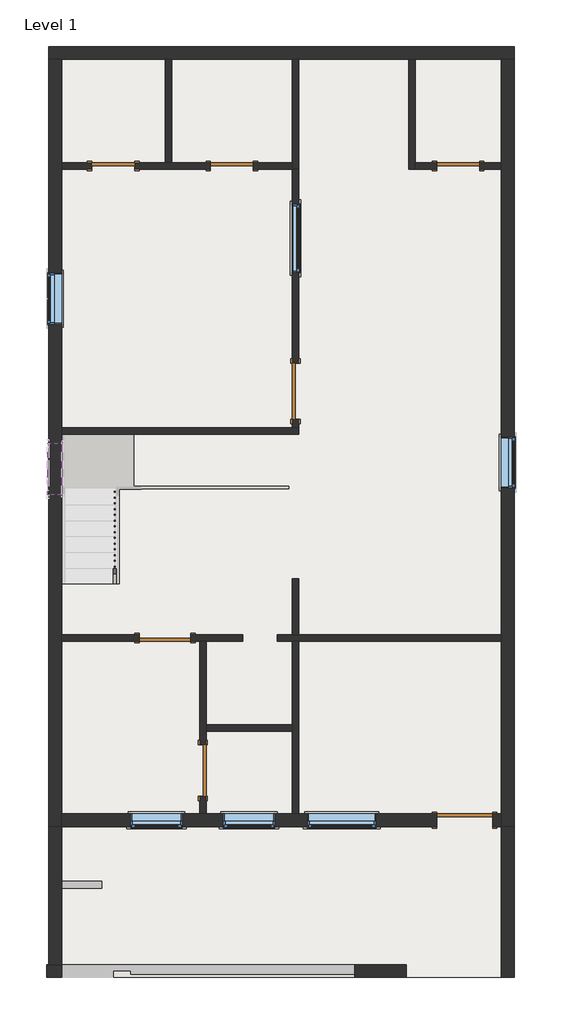
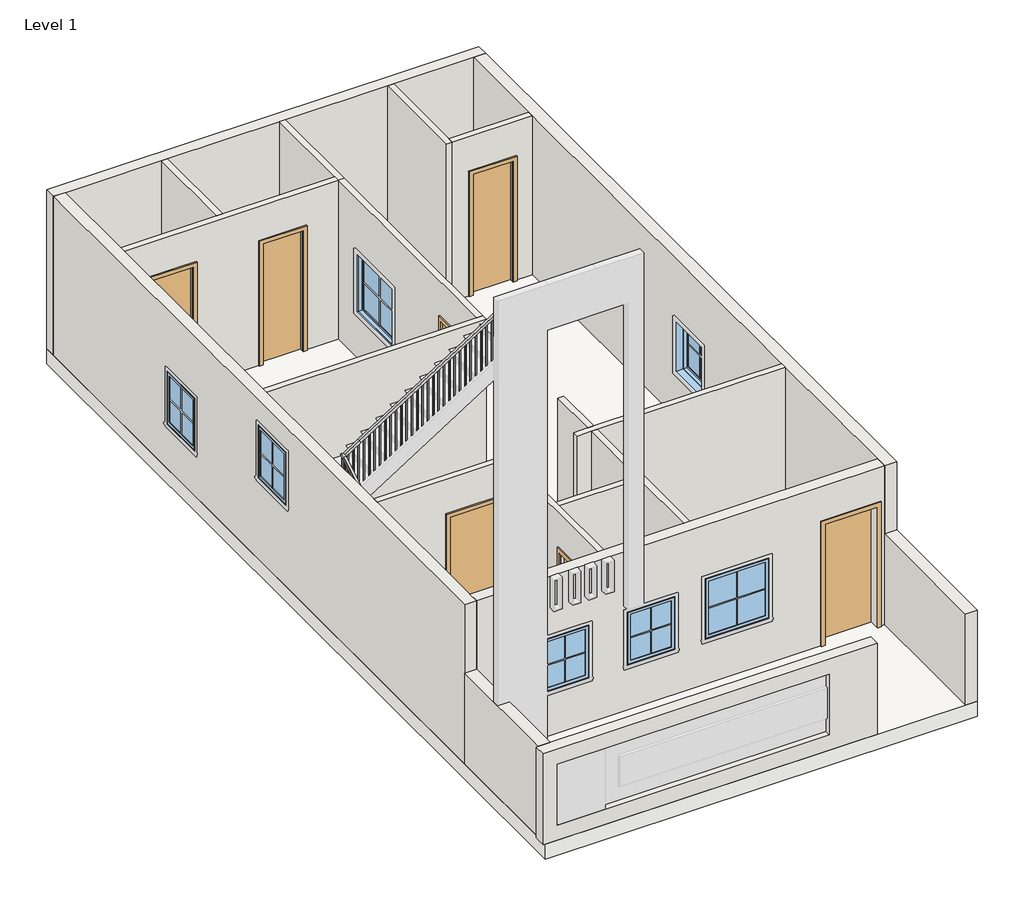
# One storey, part 1 of 2: 19 walls, 7 doors, 7 windows, 1 railing, 1 slab.
"""IFC4 building model written with IfcOpenShell, lengths in millimetres."""

from ifc_helpers import new_model, si_unit, frame, origin, origin_with_axes, place, context, project, spatial, polyline, outline, extrude, faceted_brep, transform, mapped, element, save
from components import door_02e7543a, door_3ddad2be, single_flush_d2_3_x_7_58d0fc15, door_c9b15bbd, door_019bc352, window_casement_single_left_w_4_x_4_e869003f, window_casement_single_left_w_4_x_4_9640c864, window_cb922c77, window_a1546d9a

model = new_model("IFC4")

# Units and contexts
model_context = context("Model", 3, world=origin())
ifc_project = project(units=[si_unit("LENGTHUNIT", "METRE", prefix="MILLI")], contexts=[model_context])

# Site, building, storey
site = spatial("IfcSite", under=ifc_project)
building = spatial("IfcBuilding", under=site)
storey = spatial("IfcBuildingStorey", under=building, Name="Level 1", Elevation=0.0)

# Doors
placement = place(None, origin())
door_shape = door_02e7543a(model_context)
element("IfcDoor", 1, ObjectType="Single-Flush : D1 3'3\" X 7'", at=placement, inside=storey, context=model_context, shape_type="MappedRepresentation", body=[
    mapped(door_shape, transform((-6568.6167709, -3138.8637867, 0.0), x_axis=(1.0, 0.0, 0.0), y_axis=(0.0, 1.0, 0.0), z_axis=(0.0, 0.0, 1.0))),
])
door_2_shape = door_3ddad2be(model_context)
element("IfcDoor", 2, ObjectType="Single-Flush : D1 3'3\" X 7'", at=placement, inside=storey, context=model_context, shape_type="MappedRepresentation", body=[
    mapped(door_2_shape, transform((-9559.4667709, 4443.0362133, 0.0), x_axis=(0.0, -1.0, 0.0), y_axis=(1.0, 0.0, 0.0), z_axis=(0.0, 0.0, 1.0))),
])
single_flush_d2_3_x_7_shape = single_flush_d2_3_x_7_58d0fc15(model_context)
element("IfcDoor", 3, ObjectType="Single-Flush : D2 3' X 7'", at=placement, inside=storey, context=model_context, shape_type="MappedRepresentation", body=[
    mapped(single_flush_d2_3_x_7_shape, transform((-11864.5167709, 80.5862133, 0.0), x_axis=(1.0, 0.0, 0.0), y_axis=(0.0, 1.0, 0.0), z_axis=(0.0, 0.0, 1.0))),
])
element("IfcDoor", 4, ObjectType="Single-Flush : D2 3' X 7'", at=placement, inside=storey, context=model_context, shape_type="MappedRepresentation", body=[
    mapped(single_flush_d2_3_x_7_shape, transform((-11197.7667709, -2262.5637867, 0.0), x_axis=(0.0, 1.0, 0.0), y_axis=(-1.0, 0.0, 0.0), z_axis=(0.0, 0.0, 1.0))),
])
door_3_shape = door_c9b15bbd(model_context)
element("IfcDoor", 5, ObjectType="Single-Flush : D3 2'6\" X 7'", at=placement, inside=storey, context=model_context, shape_type="MappedRepresentation", body=[
    mapped(door_3_shape, transform((-12778.9167709, 8424.4862133, 0.0), x_axis=(1.0, 0.0, 0.0), y_axis=(0.0, 1.0, 0.0), z_axis=(0.0, 0.0, 1.0))),
])
door_4_shape = door_019bc352(model_context)
element("IfcDoor", 6, ObjectType="Single-Flush : D3 2'6\" X 7'", at=placement, inside=storey, context=model_context, shape_type="MappedRepresentation", body=[
    mapped(door_4_shape, transform((-10683.4167709, 8424.4862133, 0.0), x_axis=(-1.0, 0.0, 0.0), y_axis=(0.0, -1.0, 0.0), z_axis=(0.0, 0.0, 1.0))),
])
element("IfcDoor", 7, ObjectType="Single-Flush : D3 2'6\" X 7'", at=placement, inside=storey, context=model_context, shape_type="MappedRepresentation", body=[
    mapped(door_4_shape, transform((-6682.9167709, 8424.4862133, 0.0), x_axis=(-1.0, 0.0, 0.0), y_axis=(0.0, -1.0, 0.0), z_axis=(0.0, 0.0, 1.0))),
])

# Railing
element("IfcRailing", 8, ObjectType="Handrail - Rectangular", at=placement, inside=storey, context=model_context, shape_type="SolidModel", body=[
    faceted_brep([(-12778.9167709, 1039.4362133, 1092.2), (-12778.9167709, 1039.4362133, 1031.986276), (-12728.1167709, 1039.4362133, 1031.986276), (-12728.1167709, 1039.4362133, 1092.2), (-12778.9167709, 2715.8362133, 2159.0), (-12778.9167709, 2730.6292082, 2108.2), (-12728.1167709, 2730.6292082, 2108.2), (-12728.1167709, 2715.8362133, 2159.0), (-12778.9167709, 2817.4362133, 2159.0), (-12728.1167709, 2817.4362133, 2159.0), (-12728.1167709, 2817.4362133, 2108.2), (-12778.9167709, 2817.4362133, 2108.2)], [[[0, 1, 2, 3]], [[1, 0, 4, 5]], [[2, 1, 5, 6]], [[3, 2, 6, 7]], [[0, 3, 7, 4]], [[8, 9, 10, 11]], [[5, 4, 8, 11]], [[6, 5, 11, 10]], [[7, 6, 10, 9]], [[4, 7, 9, 8]]]),
    faceted_brep([(-12728.1167709, 2817.4362133, 2159.0), (-12728.1167709, 2817.4362133, 2098.786276), (-12728.1167709, 2766.6362133, 2098.786276), (-12728.1167709, 2766.6362133, 2159.0), (-12448.7167709, 2817.4362133, 2336.8), (-12421.4434959, 2817.4362133, 2293.9419964), (-12421.4434959, 2766.6362133, 2293.9419964), (-12448.7167709, 2766.6362133, 2336.8), (-9654.7167709, 2817.4362133, 4114.8), (-9654.7167709, 2766.6362133, 4114.8), (-9654.7167709, 2766.6362133, 4054.586276), (-9654.7167709, 2817.4362133, 4054.586276)], [[[0, 1, 2, 3]], [[1, 0, 4, 5]], [[2, 1, 5, 6]], [[3, 2, 6, 7]], [[0, 3, 7, 4]], [[8, 9, 10, 11]], [[5, 4, 8, 11]], [[6, 5, 11, 10]], [[7, 6, 10, 9]], [[4, 7, 9, 8]]]),
    extrude(outline(polyline([(4028.3203669, -9695.9917709), (4016.1976396, -9715.0417709), (3022.6, -9715.0417709), (3022.6, -9695.9917709), (4028.3203669, -9695.9917709)])), frame((0.0, 2782.5112133, 0.0), z_axis=(0.0, 1.0, 0.0), x_axis=(0.0, 0.0, 1.0)), (0.0, 0.0, 1.0), 19.05),
    extrude(outline(polyline([(3963.6658214, -9797.5917709), (3951.5430941, -9816.6417709), (3022.6, -9816.6417709), (3022.6, -9797.5917709), (3963.6658214, -9797.5917709)])), frame((0.0, 2782.5112133, 0.0), z_axis=(0.0, 1.0, 0.0), x_axis=(0.0, 0.0, 1.0)), (0.0, 0.0, 1.0), 19.05),
    extrude(outline(polyline([(3899.011276, -9899.1917709), (3886.8885487, -9918.2417709), (3022.6, -9918.2417709), (3022.6, -9899.1917709), (3899.011276, -9899.1917709)])), frame((0.0, 2782.5112133, 0.0), z_axis=(0.0, 1.0, 0.0), x_axis=(0.0, 0.0, 1.0)), (0.0, 0.0, 1.0), 19.05),
    extrude(outline(polyline([(3834.3567305, -10000.7917709), (3822.2340032, -10019.8417709), (2844.8, -10019.8417709), (2844.8, -10000.7917709), (3834.3567305, -10000.7917709)])), frame((0.0, 2782.5112133, 0.0), z_axis=(0.0, 1.0, 0.0), x_axis=(0.0, 0.0, 1.0)), (0.0, 0.0, 1.0), 19.05),
    extrude(outline(polyline([(3769.7021851, -10102.3917709), (3757.5794578, -10121.4417709), (2844.8, -10121.4417709), (2844.8, -10102.3917709), (3769.7021851, -10102.3917709)])), frame((0.0, 2782.5112133, 0.0), z_axis=(0.0, 1.0, 0.0), x_axis=(0.0, 0.0, 1.0)), (0.0, 0.0, 1.0), 19.05),
    extrude(outline(polyline([(3705.0476396, -10203.9917709), (3692.9249123, -10223.0417709), (2844.8, -10223.0417709), (2844.8, -10203.9917709), (3705.0476396, -10203.9917709)])), frame((0.0, 2782.5112133, 0.0), z_axis=(0.0, 1.0, 0.0), x_axis=(0.0, 0.0, 1.0)), (0.0, 0.0, 1.0), 19.05),
    extrude(outline(polyline([(3640.3930941, -10305.5917709), (3628.2703669, -10324.6417709), (2667.0, -10324.6417709), (2667.0, -10305.5917709), (3640.3930941, -10305.5917709)])), frame((0.0, 2782.5112133, 0.0), z_axis=(0.0, 1.0, 0.0), x_axis=(0.0, 0.0, 1.0)), (0.0, 0.0, 1.0), 19.05),
    extrude(outline(polyline([(3575.7385487, -10407.1917709), (3563.6158214, -10426.2417709), (2667.0, -10426.2417709), (2667.0, -10407.1917709), (3575.7385487, -10407.1917709)])), frame((0.0, 2782.5112133, 0.0), z_axis=(0.0, 1.0, 0.0), x_axis=(0.0, 0.0, 1.0)), (0.0, 0.0, 1.0), 19.05),
    extrude(outline(polyline([(3511.0840032, -10508.7917709), (3498.961276, -10527.8417709), (2489.2, -10527.8417709), (2489.2, -10508.7917709), (3511.0840032, -10508.7917709)])), frame((0.0, 2782.5112133, 0.0), z_axis=(0.0, 1.0, 0.0), x_axis=(0.0, 0.0, 1.0)), (0.0, 0.0, 1.0), 19.05),
    extrude(outline(polyline([(3446.4294578, -10610.3917709), (3434.3067305, -10629.4417709), (2489.2, -10629.4417709), (2489.2, -10610.3917709), (3446.4294578, -10610.3917709)])), frame((0.0, 2782.5112133, 0.0), z_axis=(0.0, 1.0, 0.0), x_axis=(0.0, 0.0, 1.0)), (0.0, 0.0, 1.0), 19.05),
    extrude(outline(polyline([(3381.7749123, -10711.9917709), (3369.6521851, -10731.0417709), (2489.2, -10731.0417709), (2489.2, -10711.9917709), (3381.7749123, -10711.9917709)])), frame((0.0, 2782.5112133, 0.0), z_axis=(0.0, 1.0, 0.0), x_axis=(0.0, 0.0, 1.0)), (0.0, 0.0, 1.0), 19.05),
    extrude(outline(polyline([(3317.1203669, -10813.5917709), (3304.9976396, -10832.6417709), (2311.4, -10832.6417709), (2311.4, -10813.5917709), (3317.1203669, -10813.5917709)])), frame((0.0, 2782.5112133, 0.0), z_axis=(0.0, 1.0, 0.0), x_axis=(0.0, 0.0, 1.0)), (0.0, 0.0, 1.0), 19.05),
    extrude(outline(polyline([(3252.4658214, -10915.1917709), (3240.3430941, -10934.2417709), (2311.4, -10934.2417709), (2311.4, -10915.1917709), (3252.4658214, -10915.1917709)])), frame((0.0, 2782.5112133, 0.0), z_axis=(0.0, 1.0, 0.0), x_axis=(0.0, 0.0, 1.0)), (0.0, 0.0, 1.0), 19.05),
    extrude(outline(polyline([(3187.811276, -11016.7917709), (3175.6885487, -11035.8417709), (2311.4, -11035.8417709), (2311.4, -11016.7917709), (3187.811276, -11016.7917709)])), frame((0.0, 2782.5112133, 0.0), z_axis=(0.0, 1.0, 0.0), x_axis=(0.0, 0.0, 1.0)), (0.0, 0.0, 1.0), 19.05),
    extrude(outline(polyline([(3123.1567305, -11118.3917709), (3111.0340032, -11137.4417709), (2133.6, -11137.4417709), (2133.6, -11118.3917709), (3123.1567305, -11118.3917709)])), frame((0.0, 2782.5112133, 0.0), z_axis=(0.0, 1.0, 0.0), x_axis=(0.0, 0.0, 1.0)), (0.0, 0.0, 1.0), 19.05),
    extrude(outline(polyline([(3058.5021851, -11219.9917709), (3046.3794578, -11239.0417709), (2133.6, -11239.0417709), (2133.6, -11219.9917709), (3058.5021851, -11219.9917709)])), frame((0.0, 2782.5112133, 0.0), z_axis=(0.0, 1.0, 0.0), x_axis=(0.0, 0.0, 1.0)), (0.0, 0.0, 1.0), 19.05),
    extrude(outline(polyline([(2993.8476396, -11321.5917709), (2981.7249123, -11340.6417709), (2133.6, -11340.6417709), (2133.6, -11321.5917709), (2993.8476396, -11321.5917709)])), frame((0.0, 2782.5112133, 0.0), z_axis=(0.0, 1.0, 0.0), x_axis=(0.0, 0.0, 1.0)), (0.0, 0.0, 1.0), 19.05),
    extrude(outline(polyline([(2929.1930941, -11423.1917709), (2917.0703669, -11442.2417709), (1955.8, -11442.2417709), (1955.8, -11423.1917709), (2929.1930941, -11423.1917709)])), frame((0.0, 2782.5112133, 0.0), z_axis=(0.0, 1.0, 0.0), x_axis=(0.0, 0.0, 1.0)), (0.0, 0.0, 1.0), 19.05),
    extrude(outline(polyline([(2864.5385487, -11524.7917709), (2852.4158214, -11543.8417709), (1955.8, -11543.8417709), (1955.8, -11524.7917709), (2864.5385487, -11524.7917709)])), frame((0.0, 2782.5112133, 0.0), z_axis=(0.0, 1.0, 0.0), x_axis=(0.0, 0.0, 1.0)), (0.0, 0.0, 1.0), 19.05),
    extrude(outline(polyline([(2799.8840032, -11626.3917709), (2787.761276, -11645.4417709), (1778.0, -11645.4417709), (1778.0, -11626.3917709), (2799.8840032, -11626.3917709)])), frame((0.0, 2782.5112133, 0.0), z_axis=(0.0, 1.0, 0.0), x_axis=(0.0, 0.0, 1.0)), (0.0, 0.0, 1.0), 19.05),
    extrude(outline(polyline([(2735.2294578, -11727.9917709), (2723.1067305, -11747.0417709), (1778.0, -11747.0417709), (1778.0, -11727.9917709), (2735.2294578, -11727.9917709)])), frame((0.0, 2782.5112133, 0.0), z_axis=(0.0, 1.0, 0.0), x_axis=(0.0, 0.0, 1.0)), (0.0, 0.0, 1.0), 19.05),
    extrude(outline(polyline([(2670.5749123, -11829.5917709), (2658.4521851, -11848.6417709), (1778.0, -11848.6417709), (1778.0, -11829.5917709), (2670.5749123, -11829.5917709)])), frame((0.0, 2782.5112133, 0.0), z_axis=(0.0, 1.0, 0.0), x_axis=(0.0, 0.0, 1.0)), (0.0, 0.0, 1.0), 19.05),
    extrude(outline(polyline([(2605.9203669, -11931.1917709), (2593.7976396, -11950.2417709), (1600.2, -11950.2417709), (1600.2, -11931.1917709), (2605.9203669, -11931.1917709)])), frame((0.0, 2782.5112133, 0.0), z_axis=(0.0, 1.0, 0.0), x_axis=(0.0, 0.0, 1.0)), (0.0, 0.0, 1.0), 19.05),
    extrude(outline(polyline([(2541.2658214, -12032.7917709), (2529.1430941, -12051.8417709), (1600.2, -12051.8417709), (1600.2, -12032.7917709), (2541.2658214, -12032.7917709)])), frame((0.0, 2782.5112133, 0.0), z_axis=(0.0, 1.0, 0.0), x_axis=(0.0, 0.0, 1.0)), (0.0, 0.0, 1.0), 19.05),
    extrude(outline(polyline([(2476.611276, -12134.3917709), (2464.4885487, -12153.4417709), (1600.2, -12153.4417709), (1600.2, -12134.3917709), (2476.611276, -12134.3917709)])), frame((0.0, 2782.5112133, 0.0), z_axis=(0.0, 1.0, 0.0), x_axis=(0.0, 0.0, 1.0)), (0.0, 0.0, 1.0), 19.05),
    extrude(outline(polyline([(2411.9567305, -12235.9917709), (2399.8340032, -12255.0417709), (1422.4, -12255.0417709), (1422.4, -12235.9917709), (2411.9567305, -12235.9917709)])), frame((0.0, 2782.5112133, 0.0), z_axis=(0.0, 1.0, 0.0), x_axis=(0.0, 0.0, 1.0)), (0.0, 0.0, 1.0), 19.05),
    extrude(outline(polyline([(2347.3021851, -12337.5917709), (2335.1794578, -12356.6417709), (1422.4, -12356.6417709), (1422.4, -12337.5917709), (2347.3021851, -12337.5917709)])), frame((0.0, 2782.5112133, 0.0), z_axis=(0.0, 1.0, 0.0), x_axis=(0.0, 0.0, 1.0)), (0.0, 0.0, 1.0), 19.05),
    extrude(outline(polyline([(2217.9930941, -12540.7917709), (2205.8703669, -12559.8417709), (1244.6, -12559.8417709), (1244.6, -12540.7917709), (2217.9930941, -12540.7917709)])), frame((0.0, 2782.5112133, 0.0), z_axis=(0.0, 1.0, 0.0), x_axis=(0.0, 0.0, 1.0)), (0.0, 0.0, 1.0), 19.05),
    extrude(outline(polyline([(2153.3385487, -12642.3917709), (2141.2158214, -12661.4417709), (1244.6, -12661.4417709), (1244.6, -12642.3917709), (2153.3385487, -12642.3917709)])), frame((0.0, 2782.5112133, 0.0), z_axis=(0.0, 1.0, 0.0), x_axis=(0.0, 0.0, 1.0)), (0.0, 0.0, 1.0), 19.05),
    extrude(outline(polyline([(2655.5112133, 2060.3976396), (2674.5612133, 2072.5203669), (2674.5612133, 1066.8), (2655.5112133, 1066.8), (2655.5112133, 2060.3976396)])), frame((-12763.0417709, 0.0, 0.0), z_axis=(1.0, 0.0, 0.0), x_axis=(0.0, 1.0, 0.0)), (0.0, 0.0, 1.0), 19.05),
    extrude(outline(polyline([(2553.9112133, 1995.7430941), (2572.9612133, 2007.8658214), (2572.9612133, 1066.8), (2553.9112133, 1066.8), (2553.9112133, 1995.7430941)])), frame((-12763.0417709, 0.0, 0.0), z_axis=(1.0, 0.0, 0.0), x_axis=(0.0, 1.0, 0.0)), (0.0, 0.0, 1.0), 19.05),
    extrude(outline(polyline([(2452.3112133, 1931.0885487), (2471.3612133, 1943.211276), (2471.3612133, 1066.8), (2452.3112133, 1066.8), (2452.3112133, 1931.0885487)])), frame((-12763.0417709, 0.0, 0.0), z_axis=(1.0, 0.0, 0.0), x_axis=(0.0, 1.0, 0.0)), (0.0, 0.0, 1.0), 19.05),
    extrude(outline(polyline([(2350.7112133, 1866.4340032), (2369.7612133, 1878.5567305), (2369.7612133, 889.0), (2350.7112133, 889.0), (2350.7112133, 1866.4340032)])), frame((-12763.0417709, 0.0, 0.0), z_axis=(1.0, 0.0, 0.0), x_axis=(0.0, 1.0, 0.0)), (0.0, 0.0, 1.0), 19.05),
    extrude(outline(polyline([(2249.1112133, 1801.7794578), (2268.1612133, 1813.9021851), (2268.1612133, 889.0), (2249.1112133, 889.0), (2249.1112133, 1801.7794578)])), frame((-12763.0417709, 0.0, 0.0), z_axis=(1.0, 0.0, 0.0), x_axis=(0.0, 1.0, 0.0)), (0.0, 0.0, 1.0), 19.05),
    extrude(outline(polyline([(2147.5112133, 1737.1249123), (2166.5612133, 1749.2476396), (2166.5612133, 889.0), (2147.5112133, 889.0), (2147.5112133, 1737.1249123)])), frame((-12763.0417709, 0.0, 0.0), z_axis=(1.0, 0.0, 0.0), x_axis=(0.0, 1.0, 0.0)), (0.0, 0.0, 1.0), 19.05),
    extrude(outline(polyline([(2045.9112133, 1672.4703669), (2064.9612133, 1684.5930941), (2064.9612133, 711.2), (2045.9112133, 711.2), (2045.9112133, 1672.4703669)])), frame((-12763.0417709, 0.0, 0.0), z_axis=(1.0, 0.0, 0.0), x_axis=(0.0, 1.0, 0.0)), (0.0, 0.0, 1.0), 19.05),
    extrude(outline(polyline([(1944.3112133, 1607.8158214), (1963.3612133, 1619.9385487), (1963.3612133, 711.2), (1944.3112133, 711.2), (1944.3112133, 1607.8158214)])), frame((-12763.0417709, 0.0, 0.0), z_axis=(1.0, 0.0, 0.0), x_axis=(0.0, 1.0, 0.0)), (0.0, 0.0, 1.0), 19.05),
    extrude(outline(polyline([(1842.7112133, 1543.161276), (1861.7612133, 1555.2840032), (1861.7612133, 533.4), (1842.7112133, 533.4), (1842.7112133, 1543.161276)])), frame((-12763.0417709, 0.0, 0.0), z_axis=(1.0, 0.0, 0.0), x_axis=(0.0, 1.0, 0.0)), (0.0, 0.0, 1.0), 19.05),
    extrude(outline(polyline([(1741.1112133, 1478.5067305), (1760.1612133, 1490.6294578), (1760.1612133, 533.4), (1741.1112133, 533.4), (1741.1112133, 1478.5067305)])), frame((-12763.0417709, 0.0, 0.0), z_axis=(1.0, 0.0, 0.0), x_axis=(0.0, 1.0, 0.0)), (0.0, 0.0, 1.0), 19.05),
    extrude(outline(polyline([(1639.5112133, 1413.8521851), (1658.5612133, 1425.9749123), (1658.5612133, 533.4), (1639.5112133, 533.4), (1639.5112133, 1413.8521851)])), frame((-12763.0417709, 0.0, 0.0), z_axis=(1.0, 0.0, 0.0), x_axis=(0.0, 1.0, 0.0)), (0.0, 0.0, 1.0), 19.05),
    extrude(outline(polyline([(1537.9112133, 1349.1976396), (1556.9612133, 1361.3203669), (1556.9612133, 355.6), (1537.9112133, 355.6), (1537.9112133, 1349.1976396)])), frame((-12763.0417709, 0.0, 0.0), z_axis=(1.0, 0.0, 0.0), x_axis=(0.0, 1.0, 0.0)), (0.0, 0.0, 1.0), 19.05),
    extrude(outline(polyline([(1436.3112133, 1284.5430941), (1455.3612133, 1296.6658214), (1455.3612133, 355.6), (1436.3112133, 355.6), (1436.3112133, 1284.5430941)])), frame((-12763.0417709, 0.0, 0.0), z_axis=(1.0, 0.0, 0.0), x_axis=(0.0, 1.0, 0.0)), (0.0, 0.0, 1.0), 19.05),
    extrude(outline(polyline([(1334.7112133, 1219.8885487), (1353.7612133, 1232.011276), (1353.7612133, 355.6), (1334.7112133, 355.6), (1334.7112133, 1219.8885487)])), frame((-12763.0417709, 0.0, 0.0), z_axis=(1.0, 0.0, 0.0), x_axis=(0.0, 1.0, 0.0)), (0.0, 0.0, 1.0), 19.05),
    extrude(outline(polyline([(1233.1112133, 1155.2340032), (1252.1612133, 1167.3567305), (1252.1612133, 177.8), (1233.1112133, 177.8), (1233.1112133, 1155.2340032)])), frame((-12763.0417709, 0.0, 0.0), z_axis=(1.0, 0.0, 0.0), x_axis=(0.0, 1.0, 0.0)), (0.0, 0.0, 1.0), 19.05),
    extrude(outline(polyline([(1131.5112133, 1090.5794578), (1150.5612133, 1102.7021851), (1150.5612133, 177.8), (1131.5112133, 177.8), (1131.5112133, 1090.5794578)])), frame((-12763.0417709, 0.0, 0.0), z_axis=(1.0, 0.0, 0.0), x_axis=(0.0, 1.0, 0.0)), (0.0, 0.0, 1.0), 19.05),
    extrude(outline(polyline([(2282.6476396, -12439.1917709), (2270.5249123, -12458.2417709), (1244.6, -12458.2417709), (1244.6, -12439.1917709), (2282.6476396, -12439.1917709)])), frame((0.0, 2782.5112133, 0.0), z_axis=(0.0, 1.0, 0.0), x_axis=(0.0, 0.0, 1.0)), (0.0, 0.0, 1.0), 19.05),
    extrude(outline(polyline([(-12743.9917709, 2782.5112133), (-12763.0417709, 2782.5112133), (-12763.0417709, 2801.5612133), (-12743.9917709, 2801.5612133), (-12743.9917709, 2782.5112133)])), frame((0.0, 0.0, 1244.6), z_axis=(0.0, 0.0, 1.0), x_axis=(1.0, 0.0, 0.0)), (0.0, 0.0, 1.0), 863.6),
    extrude(outline(polyline([(2706.3112133, 2092.7249123), (2725.3612133, 2104.8476396), (2725.3612133, 1244.6), (2706.3112133, 1244.6), (2706.3112133, 2092.7249123)])), frame((-12763.0417709, 0.0, 0.0), z_axis=(1.0, 0.0, 0.0), x_axis=(0.0, 1.0, 0.0)), (0.0, 0.0, 1.0), 19.05),
    extrude(outline(polyline([(4054.586276, -9654.7167709), (4042.4635487, -9673.7667709), (3022.6, -9673.7667709), (3022.6, -9654.7167709), (4054.586276, -9654.7167709)])), frame((0.0, 2782.5112133, 0.0), z_axis=(0.0, 1.0, 0.0), x_axis=(0.0, 0.0, 1.0)), (0.0, 0.0, 1.0), 19.05),
    extrude(outline(polyline([(1039.4362133, 1031.986276), (1058.4862133, 1044.1090032), (1058.4862133, 177.8), (1039.4362133, 177.8), (1039.4362133, 1031.986276)])), frame((-12763.0417709, 0.0, 0.0), z_axis=(1.0, 0.0, 0.0), x_axis=(0.0, 1.0, 0.0)), (0.0, 0.0, 1.0), 19.05),
])

# Slab
element("IfcSlab", 9, ObjectType="Generic - 12\"", at=placement, inside=storey, context=model_context, shape_type="SweptSolid", body=[
    extrude(outline(polyline([(-5692.3167709, 10539.0362133), (-5692.3167709, -5920.1637867), (-13921.9167709, -5920.1637867), (-13921.9167709, 10539.0362133), (-5692.3167709, 10539.0362133)])), frame((0.0, 0.0, -304.8), z_axis=(0.0, 0.0, 1.0), x_axis=(1.0, 0.0, 0.0)), (0.0, 0.0, 1.0), 304.8),
])

# Walls
element("IfcWall", 10, ObjectType="4.5\" inner wall", at=placement, inside=storey, context=model_context, shape_type="SweptSolid", body=[
    extrude(outline(polyline([(-11864.5167709, 8481.6362133), (-11864.5167709, 10310.4362133), (-11750.2167709, 10310.4362133), (-11750.2167709, 8481.6362133), (-11864.5167709, 8481.6362133)])), origin_with_axes(), (0.0, 0.0, 1.0), 3200.4),
])
element("IfcWall", 11, ObjectType="4.5\" inner wall", at=placement, inside=storey, context=model_context, shape_type="Brep", body=[
    faceted_brep([(-11064.4167709, 8481.6362133, 2438.4), (-11064.4167709, 8481.6362133, 0.0), (-11750.2167709, 8481.6362133, 0.0), (-11864.5167709, 8481.6362133, 0.0), (-12397.9167709, 8481.6362133, 0.0), (-12397.9167709, 8481.6362133, 2438.4), (-13159.9167709, 8481.6362133, 2438.4), (-13159.9167709, 8481.6362133, 0.0), (-13693.3167709, 8481.6362133, 0.0), (-13693.3167709, 8481.6362133, 3200.4), (-11864.5167709, 8481.6362133, 3200.4), (-11750.2167709, 8481.6362133, 3200.4), (-9616.6167709, 8481.6362133, 3200.4), (-9616.6167709, 8481.6362133, 0.0), (-10302.4167709, 8481.6362133, 0.0), (-10302.4167709, 8481.6362133, 2438.4), (-12397.9167709, 8367.3362133, 0.0), (-11064.4167709, 8367.3362133, 0.0), (-11064.4167709, 8367.3362133, 2438.4), (-10302.4167709, 8367.3362133, 2438.4), (-10302.4167709, 8367.3362133, 0.0), (-9616.6167709, 8367.3362133, 0.0), (-9616.6167709, 8367.3362133, 3200.4), (-13693.3167709, 8367.3362133, 3200.4), (-13693.3167709, 8367.3362133, 0.0), (-13159.9167709, 8367.3362133, 0.0), (-13159.9167709, 8367.3362133, 2438.4), (-12397.9167709, 8367.3362133, 2438.4)], [[[0, 1, 2, 3, 4, 5, 6, 7, 8, 9, 10, 11, 12, 13, 14, 15]], [[16, 17, 18, 19, 20, 21, 22, 23, 24, 25, 26, 27]], [[25, 24, 8, 7]], [[14, 13, 21, 20]], [[4, 3, 2, 1, 17, 16]], [[12, 11, 10, 9, 23, 22]], [[9, 8, 24, 23]], [[13, 12, 22, 21]], [[5, 4, 16, 27]], [[6, 5, 27, 26]], [[7, 6, 26, 25]], [[18, 17, 1, 0]], [[19, 18, 0, 15]], [[20, 19, 15, 14]]]),
])
element("IfcWall", 12, ObjectType="4.5\" inner wall", at=placement, inside=storey, context=model_context, shape_type="Brep", body=[
    faceted_brep([(-9616.6167709, 10310.4362133, 0.0), (-9616.6167709, 8481.6362133, 0.0), (-9616.6167709, 8367.3362133, 0.0), (-9616.6167709, 8367.3362133, 3200.4), (-9616.6167709, 8481.6362133, 3200.4), (-9616.6167709, 10310.4362133, 3200.4), (-9502.3167709, 10310.4362133, 0.0), (-9502.3167709, 10310.4362133, 3200.4), (-9502.3167709, 8367.3362133, 3200.4), (-9502.3167709, 8367.3362133, 0.0)], [[[0, 1, 2, 3, 4, 5]], [[6, 7, 8, 9]], [[2, 1, 0, 6, 9]], [[5, 4, 3, 8, 7]], [[0, 5, 7, 6]], [[3, 2, 9, 8]]]),
])
element("IfcWall", 13, ObjectType="4.5\" inner wall", at=placement, inside=storey, context=model_context, shape_type="Brep", body=[
    faceted_brep([(-13693.3167709, 3681.0362133, 0.0), (-9502.3167709, 3681.0362133, 0.0), (-9502.3167709, 3681.0362133, 3200.4), (-13693.3167709, 3681.0362133, 3200.4), (-13693.3167709, 3795.3362133, 0.0), (-13693.3167709, 3795.3362133, 3200.4), (-9616.6167709, 3795.3362133, 3200.4), (-9502.3167709, 3795.3362133, 3200.4), (-9502.3167709, 3795.3362133, 0.0), (-9616.6167709, 3795.3362133, 0.0)], [[[0, 1, 2, 3]], [[4, 5, 6, 7, 8, 9]], [[1, 0, 4, 9, 8]], [[3, 2, 7, 6, 5]], [[0, 3, 5, 4]], [[2, 1, 8, 7]]]),
])
element("IfcWall", 14, ObjectType="4.5\" inner wall", at=placement, inside=storey, context=model_context, shape_type="SweptSolid", body=[
    extrude(outline(polyline([(3947.7362133, 2438.4), (3947.7362133, 0.0), (3795.3362133, 0.0), (3795.3362133, 3200.4), (8367.3362133, 3200.4), (8367.3362133, 0.0), (4938.3362133, 0.0), (4938.3362133, 2438.4), (3947.7362133, 2438.4)]), holes=[polyline([(6538.5362133, 2133.6), (6538.5362133, 914.4), (7757.7362133, 914.4), (7757.7362133, 2133.6), (6538.5362133, 2133.6)])]), frame((-9616.6167709, 0.0, 0.0), z_axis=(1.0, 0.0, 0.0), x_axis=(0.0, 1.0, 0.0)), (0.0, 0.0, 1.0), 114.3),
])
element("IfcWall", 15, ObjectType="4.5\" inner wall", at=placement, inside=storey, context=model_context, shape_type="Brep", body=[
    faceted_brep([(-7559.2167709, 10310.4362133, 0.0), (-7559.2167709, 8367.3362133, 0.0), (-7559.2167709, 8367.3362133, 3200.4), (-7559.2167709, 10310.4362133, 3200.4), (-7444.9167709, 10310.4362133, 0.0), (-7444.9167709, 10310.4362133, 3200.4), (-7444.9167709, 8481.6362133, 3200.4), (-7444.9167709, 8367.3362133, 3200.4), (-7444.9167709, 8367.3362133, 0.0), (-7444.9167709, 8481.6362133, 0.0)], [[[0, 1, 2, 3]], [[4, 5, 6, 7, 8, 9]], [[1, 0, 4, 9, 8]], [[3, 2, 7, 6, 5]], [[0, 3, 5, 4]], [[2, 1, 8, 7]]]),
])
element("IfcWall", 16, ObjectType="4.5\" inner wall", at=placement, inside=storey, context=model_context, shape_type="SweptSolid", body=[
    extrude(outline(polyline([(0.0, -7444.9167709), (0.0, -7063.9167709), (2438.4, -7063.9167709), (2438.4, -6301.9167709), (0.0, -6301.9167709), (0.0, -5920.9167709), (3200.4, -5920.9167709), (3200.4, -7444.9167709), (0.0, -7444.9167709)])), frame((0.0, 8367.3362133, 0.0), z_axis=(0.0, 1.0, 0.0), x_axis=(0.0, 0.0, 1.0)), (0.0, 0.0, 1.0), 114.3),
])
element("IfcWall", 17, ObjectType="4.5\" inner wall", at=placement, inside=storey, context=model_context, shape_type="Brep", body=[
    faceted_brep([(-11407.3167709, 23.4362133, 2438.4), (-11407.3167709, 23.4362133, 0.0), (-11254.9167709, 23.4362133, 0.0), (-11140.6167709, 23.4362133, 0.0), (-10492.9167709, 23.4362133, 0.0), (-10492.9167709, 23.4362133, 3200.4), (-11140.6167709, 23.4362133, 3200.4), (-11254.9167709, 23.4362133, 3200.4), (-13693.3167709, 23.4362133, 3200.4), (-13693.3167709, 23.4362133, 0.0), (-12321.7167709, 23.4362133, 0.0), (-12321.7167709, 23.4362133, 2438.4), (-10492.9167709, 137.7362133, 0.0), (-11407.3167709, 137.7362133, 0.0), (-11407.3167709, 137.7362133, 2438.4), (-12321.7167709, 137.7362133, 2438.4), (-12321.7167709, 137.7362133, 0.0), (-13693.3167709, 137.7362133, 0.0), (-13693.3167709, 137.7362133, 3200.4), (-10492.9167709, 137.7362133, 3200.4)], [[[0, 1, 2, 3, 4, 5, 6, 7, 8, 9, 10, 11]], [[12, 13, 14, 15, 16, 17, 18, 19]], [[10, 9, 17, 16]], [[4, 3, 2, 1, 13, 12]], [[5, 4, 12, 19]], [[8, 7, 6, 5, 19, 18]], [[9, 8, 18, 17]], [[14, 13, 1, 0]], [[15, 14, 0, 11]], [[16, 15, 11, 10]]]),
])
element("IfcWall", 18, ObjectType="4.5\" inner wall", at=placement, inside=storey, context=model_context, shape_type="Brep", body=[
    faceted_brep([(-11254.9167709, 23.4362133, 0.0), (-11254.9167709, -1805.3637867, 0.0), (-11254.9167709, -1805.3637867, 2438.4), (-11254.9167709, -2719.7637867, 2438.4), (-11254.9167709, -2719.7637867, 0.0), (-11254.9167709, -3024.5637867, 0.0), (-11254.9167709, -3024.5637867, 3200.4), (-11254.9167709, 23.4362133, 3200.4), (-11140.6167709, -1805.3637867, 2438.4), (-11140.6167709, -1805.3637867, 0.0), (-11140.6167709, -1564.0637867, 0.0), (-11140.6167709, -1449.7637867, 0.0), (-11140.6167709, 23.4362133, 0.0), (-11140.6167709, 23.4362133, 3200.4), (-11140.6167709, -1449.7637867, 3200.4), (-11140.6167709, -1564.0637867, 3200.4), (-11140.6167709, -3024.5637867, 3200.4), (-11140.6167709, -3024.5637867, 0.0), (-11140.6167709, -2719.7637867, 0.0), (-11140.6167709, -2719.7637867, 2438.4)], [[[0, 1, 2, 3, 4, 5, 6, 7]], [[8, 9, 10, 11, 12, 13, 14, 15, 16, 17, 18, 19]], [[18, 17, 5, 4]], [[12, 11, 10, 9, 1, 0]], [[7, 6, 16, 15, 14, 13]], [[6, 5, 17, 16]], [[0, 7, 13, 12]], [[2, 1, 9, 8]], [[3, 2, 8, 19]], [[4, 3, 19, 18]]]),
])
element("IfcWall", 19, ObjectType="4.5\" inner wall", at=placement, inside=storey, context=model_context, shape_type="Brep", body=[
    faceted_brep([(-9502.3167709, 1128.3362133, 0.0), (-9502.3167709, 1128.3362133, 3200.4), (-9502.3167709, 137.7362133, 3200.4), (-9502.3167709, 137.7362133, 0.0), (-9616.6167709, 1128.3362133, 3200.4), (-9616.6167709, 1128.3362133, 0.0), (-9616.6167709, 137.7362133, 0.0), (-9616.6167709, 137.7362133, 3200.4)], [[[0, 1, 2, 3]], [[4, 5, 6, 7]], [[5, 0, 3, 6]], [[1, 0, 5, 4]], [[1, 4, 7, 2]], [[3, 2, 7, 6]]]),
    faceted_brep([(-9502.3167709, -3024.5637867, 3200.4), (-9502.3167709, -3024.5637867, 0.0), (-9502.3167709, 23.4362133, 0.0), (-9502.3167709, 23.4362133, 3200.4), (-9616.6167709, -3024.5637867, 0.0), (-9616.6167709, -3024.5637867, 3200.4), (-9616.6167709, -1564.0637867, 3200.4), (-9616.6167709, -1449.7637867, 3200.4), (-9616.6167709, 23.4362133, 3200.4), (-9616.6167709, 23.4362133, 0.0), (-9616.6167709, -1449.7637867, 0.0), (-9616.6167709, -1564.0637867, 0.0)], [[[0, 1, 2, 3]], [[4, 5, 6, 7, 8, 9, 10, 11]], [[1, 4, 11, 10, 9, 2]], [[5, 0, 3, 8, 7, 6]], [[1, 0, 5, 4]], [[3, 2, 9, 8]]]),
])
element("IfcWall", 20, ObjectType="4.5\" inner wall", at=placement, inside=storey, context=model_context, shape_type="SweptSolid", body=[
    extrude(outline(polyline([(-9616.6167709, -1564.0637867), (-11140.6167709, -1564.0637867), (-11140.6167709, -1449.7637867), (-9616.6167709, -1449.7637867), (-9616.6167709, -1564.0637867)])), origin_with_axes(), (0.0, 0.0, 1.0), 3200.4),
])
element("IfcWall", 21, ObjectType="4.5\" inner wall", at=placement, inside=storey, context=model_context, shape_type="Brep", body=[
    faceted_brep([(-9883.3167709, 23.4362133, 0.0), (-9616.6167709, 23.4362133, 0.0), (-9502.3167709, 23.4362133, 0.0), (-5920.9167709, 23.4362133, 0.0), (-5920.9167709, 23.4362133, 3200.4), (-9502.3167709, 23.4362133, 3200.4), (-9616.6167709, 23.4362133, 3200.4), (-9883.3167709, 23.4362133, 3200.4), (-9883.3167709, 137.7362133, 0.0), (-9883.3167709, 137.7362133, 3200.4), (-9616.6167709, 137.7362133, 3200.4), (-9502.3167709, 137.7362133, 3200.4), (-5920.9167709, 137.7362133, 3200.4), (-5920.9167709, 137.7362133, 0.0), (-9502.3167709, 137.7362133, 0.0), (-9616.6167709, 137.7362133, 0.0)], [[[0, 1, 2, 3, 4, 5, 6, 7]], [[8, 9, 10, 11, 12, 13, 14, 15]], [[3, 2, 1, 0, 8, 15, 14, 13]], [[7, 6, 5, 4, 12, 11, 10, 9]], [[0, 7, 9, 8]], [[4, 3, 13, 12]]]),
])
element("IfcWall", 22, ObjectType="9\" outer wall", at=placement, inside=storey, context=model_context, shape_type="Brep", body=[
    faceted_brep([(-13921.9167709, 10310.4362133, 0.0), (-13693.3167709, 10310.4362133, 0.0), (-11864.5167709, 10310.4362133, 0.0), (-11750.2167709, 10310.4362133, 0.0), (-9616.6167709, 10310.4362133, 0.0), (-9502.3167709, 10310.4362133, 0.0), (-7559.2167709, 10310.4362133, 0.0), (-7444.9167709, 10310.4362133, 0.0), (-5920.9167709, 10310.4362133, 0.0), (-5692.3167709, 10310.4362133, 0.0), (-5692.3167709, 10310.4362133, 3200.4), (-5920.9167709, 10310.4362133, 3200.4), (-7444.9167709, 10310.4362133, 3200.4), (-7559.2167709, 10310.4362133, 3200.4), (-9502.3167709, 10310.4362133, 3200.4), (-9616.6167709, 10310.4362133, 3200.4), (-11750.2167709, 10310.4362133, 3200.4), (-11864.5167709, 10310.4362133, 3200.4), (-13693.3167709, 10310.4362133, 3200.4), (-13921.9167709, 10310.4362133, 3200.4), (-13921.9167709, 10539.0362133, 0.0), (-13921.9167709, 10539.0362133, 3200.4), (-5692.3167709, 10539.0362133, 3200.4), (-5692.3167709, 10539.0362133, 0.0)], [[[0, 1, 2, 3, 4, 5, 6, 7, 8, 9, 10, 11, 12, 13, 14, 15, 16, 17, 18, 19]], [[20, 21, 22, 23]], [[9, 8, 7, 6, 5, 4, 3, 2, 1, 0, 20, 23]], [[19, 18, 17, 16, 15, 14, 13, 12, 11, 10, 22, 21]], [[10, 9, 23, 22]], [[0, 19, 21, 20]]]),
])
element("IfcWall", 23, ObjectType="9\" outer wall", at=placement, inside=storey, context=model_context, shape_type="Brep", body=[
    faceted_brep([(-5920.9167709, 10310.4362133, 0.0), (-5920.9167709, 8481.6362133, 0.0), (-5920.9167709, 8367.3362133, 0.0), (-5920.9167709, 137.7362133, 0.0), (-5920.9167709, 23.4362133, 0.0), (-5920.9167709, -3024.5637867, 0.0), (-5920.9167709, -3253.1637867, 0.0), (-5920.9167709, -3253.1637867, 1828.8), (-5920.9167709, -3253.1637867, 3200.4), (-5920.9167709, -3024.5637867, 3200.4), (-5920.9167709, 23.4362133, 3200.4), (-5920.9167709, 137.7362133, 3200.4), (-5920.9167709, 8367.3362133, 3200.4), (-5920.9167709, 8481.6362133, 3200.4), (-5920.9167709, 10310.4362133, 3200.4), (-5920.9167709, 2728.5362133, 1981.2), (-5920.9167709, 2728.5362133, 914.4), (-5920.9167709, 3642.9362133, 914.4), (-5920.9167709, 3642.9362133, 1981.2), (-5692.3167709, 10310.4362133, 0.0), (-5692.3167709, 10310.4362133, 3200.4), (-5692.3167709, -3253.1637867, 3200.4), (-5692.3167709, -3253.1637867, 1828.8), (-5692.3167709, -3253.1637867, 0.0), (-5692.3167709, 2728.5362133, 1981.2), (-5692.3167709, 3642.9362133, 1981.2), (-5692.3167709, 3642.9362133, 914.4), (-5692.3167709, 2728.5362133, 914.4)], [[[0, 1, 2, 3, 4, 5, 6, 7, 8, 9, 10, 11, 12, 13, 14], [15, 16, 17, 18]], [[19, 20, 21, 22, 23], [24, 25, 26, 27]], [[6, 5, 4, 3, 2, 1, 0, 19, 23]], [[14, 13, 12, 11, 10, 9, 8, 21, 20]], [[0, 14, 20, 19]], [[6, 23, 22, 21, 8, 7]], [[16, 15, 24, 27]], [[17, 16, 27, 26]], [[18, 17, 26, 25]], [[15, 18, 25, 24]]]),
])
element("IfcWall", 24, ObjectType="9\" outer wall", at=placement, inside=storey, context=model_context, shape_type="Brep", body=[
    faceted_brep([(-13693.3167709, -3253.1637867, 0.0), (-13693.3167709, -3024.5637867, 0.0), (-13693.3167709, 23.4362133, 0.0), (-13693.3167709, 137.7362133, 0.0), (-13693.3167709, 3681.0362133, 0.0), (-13693.3167709, 3795.3362133, 0.0), (-13693.3167709, 8367.3362133, 0.0), (-13693.3167709, 8481.6362133, 0.0), (-13693.3167709, 10310.4362133, 0.0), (-13693.3167709, 10310.4362133, 3200.4), (-13693.3167709, 8481.6362133, 3200.4), (-13693.3167709, 8367.3362133, 3200.4), (-13693.3167709, 3795.3362133, 3200.4), (-13693.3167709, 3681.0362133, 3200.4), (-13693.3167709, 137.7362133, 3200.4), (-13693.3167709, 23.4362133, 3200.4), (-13693.3167709, -3024.5637867, 3200.4), (-13693.3167709, -3253.1637867, 3200.4), (-13693.3167709, -3253.1637867, 1828.8), (-13693.3167709, 3528.6362133, 2720.6170763), (-13693.3167709, 3528.6362133, 1653.8170763), (-13693.3167709, 2614.2362133, 1653.8170763), (-13693.3167709, 2614.2362133, 2720.6170763), (-13693.3167709, 6538.5362133, 1981.2), (-13693.3167709, 6538.5362133, 914.4), (-13693.3167709, 5624.1362133, 914.4), (-13693.3167709, 5624.1362133, 1981.2), (-13921.9167709, -3253.1637867, 0.0), (-13921.9167709, -3253.1637867, 1828.8), (-13921.9167709, -3253.1637867, 3200.4), (-13921.9167709, 10310.4362133, 3200.4), (-13921.9167709, 10310.4362133, 0.0), (-13921.9167709, 3528.6362133, 2720.6170763), (-13921.9167709, 2614.2362133, 2720.6170763), (-13921.9167709, 2614.2362133, 1653.8170763), (-13921.9167709, 3528.6362133, 1653.8170763), (-13921.9167709, 6538.5362133, 1981.2), (-13921.9167709, 5624.1362133, 1981.2), (-13921.9167709, 5624.1362133, 914.4), (-13921.9167709, 6538.5362133, 914.4)], [[[0, 1, 2, 3, 4, 5, 6, 7, 8, 9, 10, 11, 12, 13, 14, 15, 16, 17, 18], [19, 20, 21, 22], [23, 24, 25, 26]], [[27, 28, 29, 30, 31], [32, 33, 34, 35], [36, 37, 38, 39]], [[8, 7, 6, 5, 4, 3, 2, 1, 0, 27, 31]], [[17, 16, 15, 14, 13, 12, 11, 10, 9, 30, 29]], [[0, 18, 17, 29, 28, 27]], [[9, 8, 31, 30]], [[20, 19, 32, 35]], [[21, 20, 35, 34]], [[22, 21, 34, 33]], [[19, 22, 33, 32]], [[24, 23, 36, 39]], [[25, 24, 39, 38]], [[26, 25, 38, 37]], [[23, 26, 37, 36]]]),
])
element("IfcWall", 25, ObjectType="9\" outer wall", at=placement, inside=storey, context=model_context, shape_type="Brep", body=[
    faceted_brep([(-5920.9167709, -3024.5637867, 0.0), (-6073.3167709, -3024.5637867, 0.0), (-6073.3167709, -3024.5637867, 2438.4), (-7063.9167709, -3024.5637867, 2438.4), (-7063.9167709, -3024.5637867, 0.0), (-9502.3167709, -3024.5637867, 0.0), (-9616.6167709, -3024.5637867, 0.0), (-11140.6167709, -3024.5637867, 0.0), (-11254.9167709, -3024.5637867, 0.0), (-13693.3167709, -3024.5637867, 0.0), (-13693.3167709, -3024.5637867, 3200.4), (-11254.9167709, -3024.5637867, 3200.4), (-11140.6167709, -3024.5637867, 3200.4), (-9616.6167709, -3024.5637867, 3200.4), (-9502.3167709, -3024.5637867, 3200.4), (-5920.9167709, -3024.5637867, 3200.4), (-8130.7167709, -3024.5637867, 2133.6), (-9349.9167709, -3024.5637867, 2133.6), (-9349.9167709, -3024.5637867, 914.4), (-8130.7167709, -3024.5637867, 914.4), (-9921.4167709, -3024.5637867, 1981.2), (-10835.8167709, -3024.5637867, 1981.2), (-10835.8167709, -3024.5637867, 914.4), (-9921.4167709, -3024.5637867, 914.4), (-11559.7167709, -3024.5637867, 1981.2), (-12474.1167709, -3024.5637867, 1981.2), (-12474.1167709, -3024.5637867, 914.4), (-11559.7167709, -3024.5637867, 914.4), (-6073.3167709, -3253.1637867, 2438.4), (-6073.3167709, -3253.1637867, 0.0), (-5920.9167709, -3253.1637867, 0.0), (-5920.9167709, -3253.1637867, 3200.4), (-13693.3167709, -3253.1637867, 3200.4), (-13693.3167709, -3253.1637867, 0.0), (-7063.9167709, -3253.1637867, 0.0), (-7063.9167709, -3253.1637867, 2438.4), (-8130.7167709, -3253.1637867, 2133.6), (-8130.7167709, -3253.1637867, 914.4), (-9349.9167709, -3253.1637867, 914.4), (-9349.9167709, -3253.1637867, 2133.6), (-9921.4167709, -3253.1637867, 1981.2), (-9921.4167709, -3253.1637867, 914.4), (-10835.8167709, -3253.1637867, 914.4), (-10835.8167709, -3253.1637867, 1981.2), (-11559.7167709, -3253.1637867, 1981.2), (-11559.7167709, -3253.1637867, 914.4), (-12474.1167709, -3253.1637867, 914.4), (-12474.1167709, -3253.1637867, 1981.2)], [[[0, 1, 2, 3, 4, 5, 6, 7, 8, 9, 10, 11, 12, 13, 14, 15], [16, 17, 18, 19], [20, 21, 22, 23], [24, 25, 26, 27]], [[28, 29, 30, 31, 32, 33, 34, 35], [36, 37, 38, 39], [40, 41, 42, 43], [44, 45, 46, 47]], [[34, 33, 9, 8, 7, 6, 5, 4]], [[30, 29, 1, 0]], [[15, 14, 13, 12, 11, 10, 32, 31]], [[37, 36, 16, 19]], [[38, 37, 19, 18]], [[39, 38, 18, 17]], [[36, 39, 17, 16]], [[41, 40, 20, 23]], [[42, 41, 23, 22]], [[43, 42, 22, 21]], [[40, 43, 21, 20]], [[45, 44, 24, 27]], [[46, 45, 27, 26]], [[47, 46, 26, 25]], [[44, 47, 25, 24]], [[2, 1, 29, 28]], [[3, 2, 28, 35]], [[4, 3, 35, 34]], [[9, 33, 32, 10]], [[15, 31, 30, 0]]]),
])
element("IfcWall", 26, ObjectType="9\" outer wall", at=placement, inside=storey, context=model_context, shape_type="Brep", body=[
    faceted_brep([(-7597.3167709, -5691.5637867, 0.0), (-13693.3167709, -5691.5637867, 0.0), (-13921.9167709, -5691.5637867, 0.0), (-13960.0167709, -5691.5637867, 0.0), (-13960.0167709, -5691.5637867, 1828.8), (-13921.9167709, -5691.5637867, 1828.8), (-13693.3167709, -5691.5637867, 1828.8), (-7597.3167709, -5691.5637867, 1828.8), (-8511.7167709, -5691.5637867, 1524.0), (-13693.3167709, -5691.5637867, 1524.0), (-13693.3167709, -5691.5637867, 304.8), (-8511.7167709, -5691.5637867, 304.8), (-7597.3167709, -5920.1637867, 0.0), (-7597.3167709, -5920.1637867, 1828.8), (-13960.0167709, -5920.1637867, 1828.8), (-13960.0167709, -5920.1637867, 0.0), (-8511.7167709, -5920.1637867, 1524.0), (-8511.7167709, -5920.1637867, 304.8), (-13693.3167709, -5920.1637867, 304.8), (-13693.3167709, -5920.1637867, 1524.0)], [[[0, 1, 2, 3, 4, 5, 6, 7], [8, 9, 10, 11]], [[12, 13, 14, 15], [16, 17, 18, 19]], [[3, 2, 1, 0, 12, 15]], [[7, 6, 5, 4, 14, 13]], [[0, 7, 13, 12]], [[4, 3, 15, 14]], [[9, 8, 16, 19]], [[11, 10, 18, 17]], [[8, 11, 17, 16]], [[10, 9, 19, 18]]]),
])
element("IfcWall", 27, ObjectType="9\" outer wall", at=placement, inside=storey, context=model_context, shape_type="Brep", body=[
    faceted_brep([(-13921.9167709, -3253.1637867, 0.0), (-13921.9167709, -5691.5637867, 0.0), (-13921.9167709, -5691.5637867, 1828.8), (-13921.9167709, -3253.1637867, 1828.8), (-13693.3167709, -3253.1637867, 0.0), (-13693.3167709, -3253.1637867, 1828.8), (-13693.3167709, -5691.5637867, 1828.8), (-13693.3167709, -5691.5637867, 1524.0), (-13693.3167709, -5691.5637867, 304.8), (-13693.3167709, -5691.5637867, 0.0)], [[[0, 1, 2, 3]], [[4, 5, 6, 7, 8, 9]], [[1, 0, 4, 9]], [[3, 2, 6, 5]], [[0, 3, 5, 4]], [[1, 9, 8, 7, 6, 2]]]),
])
element("IfcWall", 28, ObjectType="9\" outer wall", at=placement, inside=storey, context=model_context, shape_type="SweptSolid", body=[
    extrude(outline(polyline([(-5692.3167709, -3253.1637867), (-5692.3167709, -5920.1637867), (-5920.9167709, -5920.1637867), (-5920.9167709, -3253.1637867), (-5692.3167709, -3253.1637867)])), origin_with_axes(), (0.0, 0.0, 1.0), 1828.8),
])

# Windows
window_casement_single_left_w_4_x_4_shape = window_casement_single_left_w_4_x_4_e869003f(model_context)
element("IfcWindow", 29, ObjectType="Window-Casement-Single_Left : W 4' X 4'", at=placement, inside=storey, context=model_context, shape_type="MappedRepresentation", body=[
    mapped(window_casement_single_left_w_4_x_4_shape, transform((-8740.3167709, -3138.8637867, 0.0), x_axis=(1.0, 0.0, 0.0), y_axis=(0.0, 1.0, 0.0), z_axis=(0.0, 0.0, 1.0))),
])
window_casement_single_left_w_4_x_4_2_shape = window_casement_single_left_w_4_x_4_9640c864(model_context)
element("IfcWindow", 30, ObjectType="Window-Casement-Single_Left : W 4' X 4'", at=placement, inside=storey, context=model_context, shape_type="MappedRepresentation", body=[
    mapped(window_casement_single_left_w_4_x_4_2_shape, transform((-9559.4667709, 7148.1362133, 0.0), x_axis=(0.0, -1.0, 0.0), y_axis=(1.0, 0.0, 0.0), z_axis=(0.0, 0.0, 1.0))),
])
window_shape = window_cb922c77(model_context)
element("IfcWindow", 31, ObjectType="Window-Casement-Single_Left : W3 3' X 3'6\"", at=placement, inside=storey, context=model_context, shape_type="MappedRepresentation", body=[
    mapped(window_shape, transform((-10378.6167709, -3138.8637867, 0.0), x_axis=(1.0, 0.0, 0.0), y_axis=(0.0, 1.0, 0.0), z_axis=(0.0, 0.0, 1.0))),
])
element("IfcWindow", 32, ObjectType="Window-Casement-Single_Left : W3 3' X 3'6\"", at=placement, inside=storey, context=model_context, shape_type="MappedRepresentation", body=[
    mapped(window_shape, transform((-12016.9167709, -3138.8637867, 0.0), x_axis=(1.0, 0.0, 0.0), y_axis=(0.0, 1.0, 0.0), z_axis=(0.0, 0.0, 1.0))),
])
window_2_shape = window_a1546d9a(model_context)
element("IfcWindow", 33, ObjectType="Window-Casement-Single_Left : W3 3' X 3'6\"", at=placement, inside=storey, context=model_context, shape_type="MappedRepresentation", body=[
    mapped(window_2_shape, transform((-5806.6167709, 3185.7362133, 0.0), x_axis=(0.0, -1.0, 0.0), y_axis=(1.0, 0.0, 0.0), z_axis=(0.0, 0.0, 1.0))),
])
element("IfcWindow", 34, ObjectType="Window-Casement-Single_Left : W3 3' X 3'6\"", at=placement, inside=storey, context=model_context, shape_type="MappedRepresentation", body=[
    mapped(window_2_shape, transform((-13807.6167709, 3071.4362133, 739.4170763), x_axis=(0.0, 1.0, 0.0), y_axis=(-1.0, 0.0, 0.0), z_axis=(0.0, 0.0, 1.0))),
])
element("IfcWindow", 35, ObjectType="Window-Casement-Single_Left : W3 3' X 3'6\"", at=placement, inside=storey, context=model_context, shape_type="MappedRepresentation", body=[
    mapped(window_2_shape, transform((-13807.6167709, 6081.3362133, 0.0), x_axis=(0.0, 1.0, 0.0), y_axis=(-1.0, 0.0, 0.0), z_axis=(0.0, 0.0, 1.0))),
])

save(model, "model.ifc")

# Revit data of these elements
# Type "Single-Flush : D1 3'3\" X 7'"
#   Type Mark = "9"
#   Construction Type Id = "MDOOR"
#   Assembly Code = "C1020"
#   Analytic Construction = "Metal"
#   Thickness = 0' - 2"
#   Heat Transfer Coefficient (U) = 0.651978 BTU/(h·ft²·°F)
#   Height = 8' - 0"
#   Trim Projection Ext = 0' - 1"
#   Trim Projection Int = 0' - 1"
#   Trim Width = 0' - 3"
#   Width = 3' - 3"
#   Define Thermal Properties by = 1
#   Door Material = Door - Panel
#   Frame Material = Door - Frame
#   Visual Light Transmittance = 0
#   Solar Heat Gain Coefficient = 0
#   Function = (empty or 0)
#   Wall Closure = (empty or 0)
# Type "Single-Flush : D2 3' X 7'"
#   Type Mark = "10"
#   Construction Type Id = "MDOOR"
#   Assembly Code = "C1020"
#   Analytic Construction = "Metal"
#   Thickness = 0' - 2"
#   Heat Transfer Coefficient (U) = 0.651978 BTU/(h·ft²·°F)
#   Height = 8' - 0"
#   Trim Projection Ext = 0' - 1"
#   Trim Projection Int = 0' - 1"
#   Trim Width = 0' - 3"
#   Width = 3' - 0"
#   Define Thermal Properties by = 1
#   Door Material = Door - Panel
#   Frame Material = Door - Frame
#   Visual Light Transmittance = 0
#   Solar Heat Gain Coefficient = 0
#   Function = (empty or 0)
#   Wall Closure = (empty or 0)
# Type "Single-Flush : D3 2'6\" X 7'"
#   Type Mark = "11"
#   Construction Type Id = "MDOOR"
#   Assembly Code = "C1020"
#   Analytic Construction = "Metal"
#   Thickness = 0' - 2"
#   Heat Transfer Coefficient (U) = 0.651978 BTU/(h·ft²·°F)
#   Height = 8' - 0"
#   Trim Projection Ext = 0' - 1"
#   Trim Projection Int = 0' - 1"
#   Trim Width = 0' - 3"
#   Width = 2' - 6"
#   Define Thermal Properties by = 1
#   Door Material = Door - Panel
#   Frame Material = Door - Frame
#   Visual Light Transmittance = 0
#   Solar Heat Gain Coefficient = 0
#   Function = (empty or 0)
#   Wall Closure = (empty or 0)
# Type "Handrail - Rectangular"
#   Assembly Code = "C2010400"
#   built-in parameter 1008612 = 0.0416667 (stored number, unit not read)
#   built-in parameter 1008611 = 0.0416667 (stored number, unit not read)
#   built-in parameter 1008609 = 0.333333 (stored number, unit not read)
#   built-in parameter 1008604 = 0.166667 (stored number, unit not read)
#   built-in parameter 1008603 = 0.166667 (stored number, unit not read)
#   Railing Height = 3' - 0"
#   built-in parameter 1008630 = 2
#   built-in parameter 1008610 = 2
#   built-in parameter 1008618 = Baluster - Square : 3/4"
# Type "Generic - 12\""
#   Assembly Code = "B1010"
#   Function = 0
#   Layers, outside or top first: 1' - 0" no material (function 1)
# Type "4.5\" inner wall"
#   Assembly Code = "B2010"
#   Layers, outside or top first: 0' - 4 1/2" no material (function 1)
# Type "9\" outer wall"
#   Assembly Code = "B2010"
#   Layers, outside or top first: 0' - 9" no material (function 1)
# Type "Window-Casement-Single_Left : W 4' X 4'"
#   Type Mark = "19"
#   Fire Rating = "0.5h"
#   Assembly Code = "B2020100"
#   Analytic Construction = "Double glazing - domestic"
#   Window Inset [instance default] = 0' - 0"
#   Wall Thickness [instance default] = 0' - 6"
#   Visual Light Transmittance = 0.81
#   Thermal Resistance (R) = 1.8146 (h·ft²·°F)/BTU
#   Solar Heat Gain Coefficient = 0.76
#   Rough Width = 4' - 0 1/2"
#   Rough Height = 4' - 0 1/2"
#   Interior Wall Closure [instance default] = 0' - 2 1/4"
#   Height = 4' - 0"
#   Heat Transfer Coefficient (U) = 0.5511 BTU/(h·ft²·°F)
#   Frame Extension [instance default] = 0' - 0 1/4"
#   Exterior Wall Closure [instance default] = 0' - 1 1/4"
#   Extension Jamb [instance default] = 0' - 2 1/4"
#   Default Sill Height = 3' - 0"
#   Width = 4' - 0"
#   Muntin Visibility = yes
#   Interior Trim Visibility [instance default] = yes
#   Exterior Trim Visibility [instance default] = yes
#   Extension Jamb Visibility [instance default] = yes
#   Muntin Pattern = Muntin Pattern_2x2 : Muntin Pattern_2x2
#   Interior Trim Material = Wood - Stained
#   Interior Trim = Trim-Window-Interior-Flat : Picture Frame
#   Interior Frame Material = Wood - Stained
#   Glass Panel Material = Glass
#   Exterior Trim Material = Clad - White
#   Exterior Trim = Trim-Window-Exterior-Flat : with Sill
#   Exterior Frame Material = Clad - White
#   Wall Closure = (empty or 0)
# Type "Window-Casement-Single_Left : W3 3' X 3'6\""
#   Type Mark = "20"
#   Fire Rating = "0.5h"
#   Assembly Code = "B2020100"
#   Analytic Construction = "Double glazing - domestic"
#   Window Inset [instance default] = 0' - 0"
#   Wall Thickness [instance default] = 0' - 6"
#   Visual Light Transmittance = 0.81
#   Thermal Resistance (R) = 1.8146 (h·ft²·°F)/BTU
#   Solar Heat Gain Coefficient = 0.76
#   Rough Width = 3' - 0 1/2"
#   Rough Height = 3' - 6 1/2"
#   Interior Wall Closure [instance default] = 0' - 2 1/4"
#   Height = 3' - 6"
#   Heat Transfer Coefficient (U) = 0.5511 BTU/(h·ft²·°F)
#   Frame Extension [instance default] = 0' - 0 1/4"
#   Exterior Wall Closure [instance default] = 0' - 1 1/4"
#   Extension Jamb [instance default] = 0' - 2 1/4"
#   Default Sill Height = 3' - 0"
#   Width = 3' - 0"
#   Muntin Visibility = yes
#   Interior Trim Visibility [instance default] = yes
#   Exterior Trim Visibility [instance default] = yes
#   Extension Jamb Visibility [instance default] = yes
#   Muntin Pattern = Muntin Pattern_2x2 : Muntin Pattern_2x2
#   Interior Trim Material = Wood - Stained
#   Interior Trim = Trim-Window-Interior-Flat : Picture Frame
#   Interior Frame Material = Wood - Stained
#   Glass Panel Material = Glass
#   Exterior Trim Material = Clad - White
#   Exterior Trim = Trim-Window-Exterior-Flat : with Sill
#   Exterior Frame Material = Clad - White
#   Wall Closure = (empty or 0)
# Elements 1, 2 (IfcDoor, "Single-Flush : D1 3'3\" X 7'")
#   Phase Created = New Construction
#   Materials on its faces: "Door - Frame", "Door - Panel"
# Elements 3, 4 (IfcDoor, "Single-Flush : D2 3' X 7'")
#   Phase Created = New Construction
#   Materials on its faces: "Door - Frame", "Door - Panel"
# Elements 5, 6, 7 (IfcDoor, "Single-Flush : D3 2'6\" X 7'")
#   Phase Created = New Construction
#   Materials on its faces: "Door - Frame", "Door - Panel"
# Element 8 (IfcRailing, "Handrail - Rectangular")
#   Phase Created = New Construction
# Element 9 (IfcSlab, "Generic - 12\"")
#   Height Offset From Level = 0' - 0"
#   Phase Created = New Construction
#   Materials on its faces: "Default Floor"
# Elements 10, 11, 12, 13, 14, 15, 16, 17, 18, 19, 20, 21 (IfcWall, "4.5\" inner wall")
#   Top Offset = 0' - 0"
#   Base Offset = 0' - 0"
#   wall height = 10' - 6"
#   Phase Created = New Construction
#   Base Constraint = Level 1
#   Top Constraint = Level 2
#   Materials on its faces: "Default Wall"
# Elements 22, 23, 24, 25 (IfcWall, "9\" outer wall")
#   Top Offset = 0' - 0"
#   Base Offset = 0' - 0"
#   wall height = 10' - 6"
#   Phase Created = New Construction
#   Base Constraint = Level 1
#   Top Constraint = Level 2
#   Materials on its faces: "Default Wall"
# Elements 26, 27, 28 (IfcWall, "9\" outer wall")
#   Top Offset = 0' - 0"
#   Base Offset = 0' - 0"
#   Unconnected Height = 6' - 0"
#   wall height = 6' - 0"
#   Phase Created = New Construction
#   Base Constraint = Level 1
#   Materials on its faces: "Default Wall"
# Element 29 (IfcWindow, "Window-Casement-Single_Left : W 4' X 4'")
#   Mark = "1"
#   Window Inset = 0' - 0"
#   Interior Wall Closure = 0' - 2 1/4"
#   Frame Extension = 0' - 0 1/4"
#   Exterior Wall Closure = 0' - 1 1/4"
#   Interior Trim Visibility = yes
#   Exterior Trim Visibility = yes
#   Phase Created = New Construction
#   Materials on its faces: "Wood - Stained", "Glass", "Clad - White"
# Element 30 (IfcWindow, "Window-Casement-Single_Left : W 4' X 4'")
#   Mark = "7"
#   Window Inset = 0' - 0"
#   Interior Wall Closure = 0' - 2 1/4"
#   Frame Extension = 0' - 0 1/4"
#   Exterior Wall Closure = 0' - 1 1/4"
#   Interior Trim Visibility = yes
#   Exterior Trim Visibility = yes
#   Phase Created = New Construction
#   Materials on its faces: "Wood - Stained", "Glass", "Clad - White"
# Element 31 (IfcWindow, "Window-Casement-Single_Left : W3 3' X 3'6\"")
#   Mark = "2"
#   Window Inset = 0' - 0"
#   Interior Wall Closure = 0' - 2 1/4"
#   Frame Extension = 0' - 0 1/4"
#   Exterior Wall Closure = 0' - 1 1/4"
#   Interior Trim Visibility = yes
#   Exterior Trim Visibility = yes
#   Phase Created = New Construction
#   Materials on its faces: "Wood - Stained", "Glass", "Clad - White"
# Element 32 (IfcWindow, "Window-Casement-Single_Left : W3 3' X 3'6\"")
#   Mark = "3"
#   Window Inset = 0' - 0"
#   Interior Wall Closure = 0' - 2 1/4"
#   Frame Extension = 0' - 0 1/4"
#   Exterior Wall Closure = 0' - 1 1/4"
#   Interior Trim Visibility = yes
#   Exterior Trim Visibility = yes
#   Phase Created = New Construction
#   Materials on its faces: "Wood - Stained", "Glass", "Clad - White"
# Element 33 (IfcWindow, "Window-Casement-Single_Left : W3 3' X 3'6\"")
#   Mark = "12"
#   Window Inset = 0' - 0"
#   Interior Wall Closure = 0' - 2 1/4"
#   Frame Extension = 0' - 0 1/4"
#   Exterior Wall Closure = 0' - 1 1/4"
#   Interior Trim Visibility = yes
#   Exterior Trim Visibility = yes
#   Phase Created = New Construction
#   Materials on its faces: "Wood - Stained", "Glass", "Clad - White"
# Element 34 (IfcWindow, "Window-Casement-Single_Left : W3 3' X 3'6\"")
#   Mark = "13"
#   Window Inset = 0' - 0"
#   Interior Wall Closure = 0' - 2 1/4"
#   Frame Extension = 0' - 0 1/4"
#   Exterior Wall Closure = 0' - 1 1/4"
#   Interior Trim Visibility = yes
#   Exterior Trim Visibility = yes
#   Phase Created = New Construction
